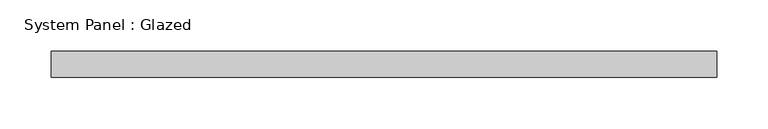
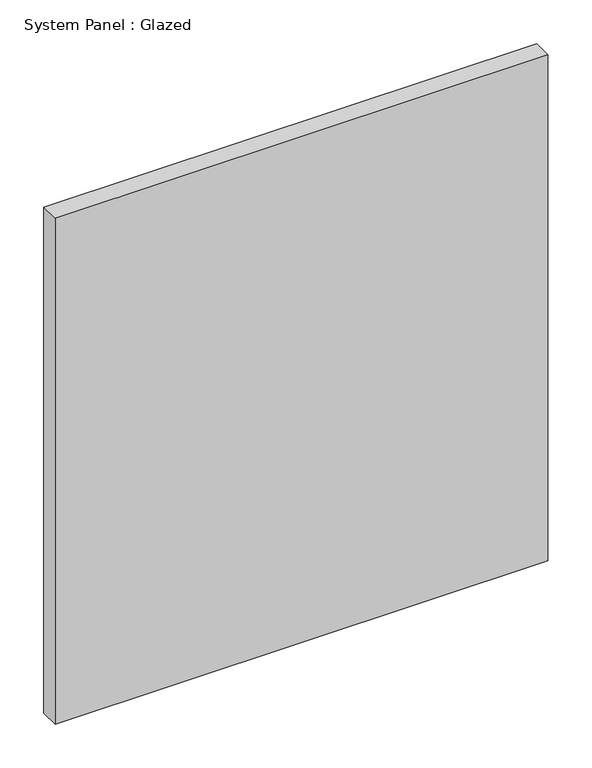
"""IFC4 building model written with IfcOpenShell, lengths in millimetres: plate geometry, System Panel : Glazed."""

from ifc_helpers import new_model, si_unit, origin, origin_with_axes, place, context, project, spatial, polyline, outline, extrude, source, transform, mapped, element, save


def system_panel_glazed_aefe9f20(model_context):
    return source(origin(), model_context, "Body", "SweptSolid", [
        extrude(outline(polyline([(323.85, 19.05), (-323.85, 19.05), (-323.85, 44.45), (323.85, 44.45), (323.85, 19.05)])), origin_with_axes(), (0.0, 0.0, 1.0), 703.2943895),
    ])


if __name__ == "__main__":
    model = new_model("IFC4")
    model_context = context("Model", 3, world=origin())
    ifc_project = project(units=[si_unit("LENGTHUNIT", "METRE", prefix="MILLI")], contexts=[model_context])
    site = spatial("IfcSite", under=ifc_project)
    building = spatial("IfcBuilding", under=site)
    placement = place(None, origin())
    system_panel_glazed_shape = system_panel_glazed_aefe9f20(model_context)
    element("IfcPlate", 1, ObjectType="System Panel : Glazed", at=placement, inside=building, context=model_context, shape_type="MappedRepresentation", body=[
        mapped(system_panel_glazed_shape, transform((0.0, 0.0, 0.0), x_axis=(1.0, 0.0, 0.0), y_axis=(0.0, 1.0, 0.0), z_axis=(0.0, 0.0, 1.0))),
    ])
    save(model, "model.ifc")

# Revit data of these elements
# Type "System Panel : Glazed"
#   Construction Type Id = "GSP4R"
#   Analytic Construction = "1/8 in Pilkington single glazing"
#   Visual Light Transmittance = 0.9
#   Solar Heat Gain Coefficient = 0.86
#   Heat Transfer Coefficient (U) = 1.18115 BTU/(h·ft²·°F)
#   Define Thermal Properties by = 1
# Element 1 (IfcPlate, "System Panel : Glazed")
#   Materials on its faces: "Glass"
# Materials
#   "Glass": class "Glass", colour RGB 0 128 192, transparency 0.75, Description = "Soda Lime Glass", Cost = 0
